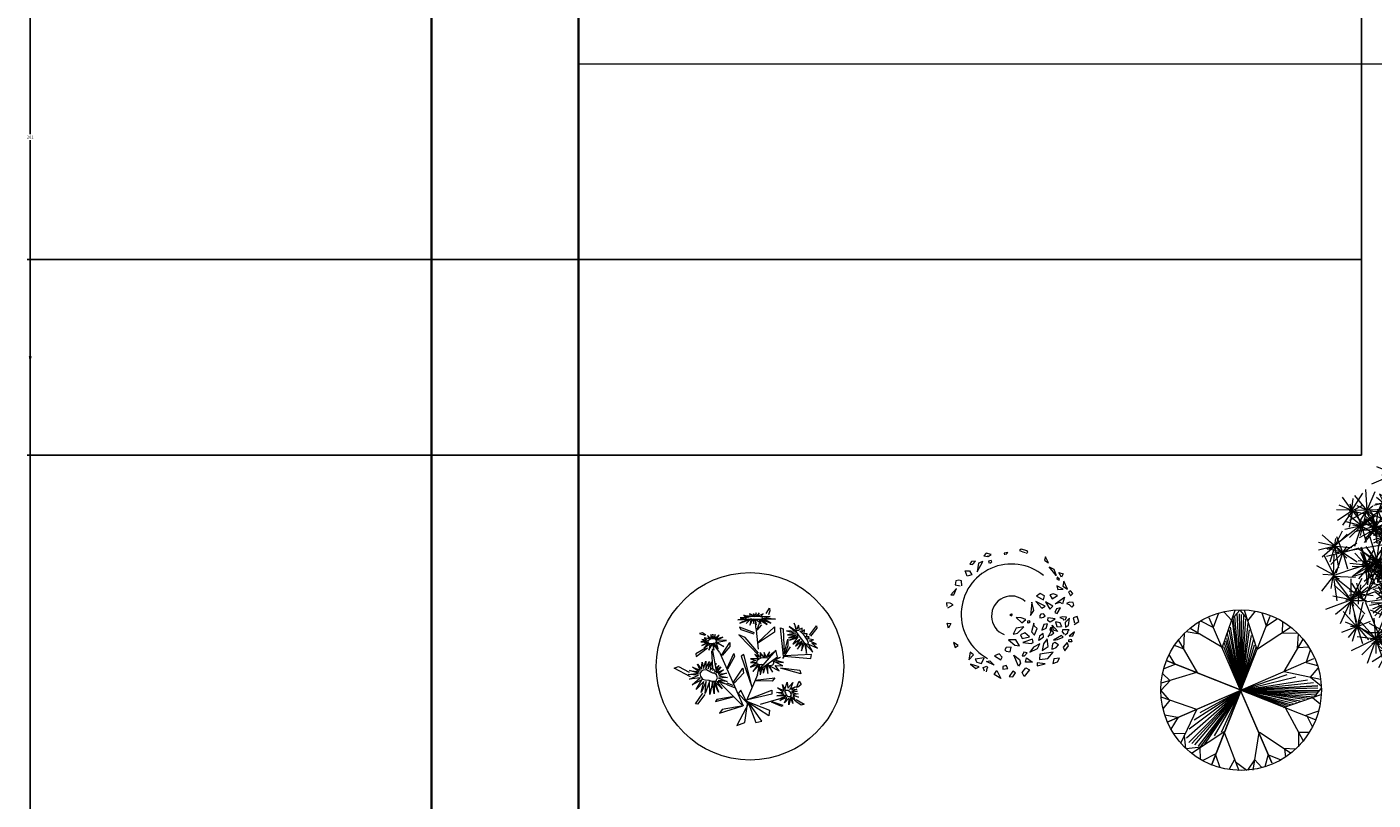
# Model space of a CAD drawing. Units: inches. Extents: x 8049 to 8459, y 820 to 1350.
# Tile 7 of 25: x 8050 to 8132, y 905 to 952. Entities that reach past the tile are written whole.
import ezdxf

# ---------------------------------------------------------------- set-up
doc = ezdxf.new("R2010")
doc.units = ezdxf.units.IN
doc.header["$MEASUREMENT"] = 0
for name, color, linetype, lineweight in [('A-ANNO-DIMS', 2, 'Continuous', 18), ('A-FLOR-STRS', 7, 'Continuous', 25), ('C-SITE-WALL', 7, 'Continuous', 35), ('L-PLNT-BEDS', 94, 'Continuous', 18), ('zelen', 69, 'Continuous', 13)]:
    doc.layers.add(name, color=color, linetype=linetype, lineweight=lineweight)
doc.styles.get("Standard").update_dxf_attribs({"font": 'arial.ttf'})
doc.dimstyles.get("Standard").update_dxf_attribs({"dimtxt": 0.18, "dimasz": 0.18, "dimexe": 0.18, "dimexo": 0.0625, "dimgap": 0.09, "dimtad": 0, "dimtih": 1, "dimtoh": 1, "dimdec": 4, "dimzin": 0, "dimdsep": 46, "dimtxsty": 'Standard', "dimcen": 0.09, "dimadec": 0, "dimazin": 0, "dimtfac": 1, "dimtdec": 4, "dimtofl": 0, "dimtmove": 0, "dimatfit": 3, "dimfxl": 1, "dimtolj": 1, "dimtzin": 0, "dimarcsym": 0})

# ---------------------------------------------------------------- blocks, each defined once
blk = doc.blocks.new('z_07')
for p, q in [((85.3, 280.8), (103, 308.6)), ((105.8, 294.2), (97.8, 273.4)), ((103, 308.6), (105.8, 294.2)), ((-21, 251.8), (-63.9, 246.3)), ((-63.9, 246.3), (-10.6, 249.9)), ((-10.6, 249.9), (-53.8, 228)), ((-53.8, 228), (-0.5, 249)), ((-17.8, 259.4), (-52, 257.4)), ((-52, 257.4), (-21, 251.8)), ((-33.4, 271.7), (-17.8, 259.4)), ((-5.4, 260.2), (-33.4, 271.7)), ((-20.7, 227.5), (5.4, 252.6)), ((-0.5, 249), (-20.7, 227.5)), ((-17.3, 268.5), (-5.4, 260.2)), ((0.4, 263.9), (-17.3, 268.5)), ((-2, 279), (0.4, 263.9)), ((16.1, 266.2), (-2, 279)), ((5.4, 252.6), (-0.2, 218.2)), ((-0.2, 218.2), (16.1, 251.8)), ((6.4, 274.5), (16.1, 266.2)), ((23.4, 266.3), (6.4, 274.5)), ((16.1, 251.8), (19.1, 227.4)), ((19, 279.6), (23.4, 266.3)), ((27.9, 266.9), (19, 279.6)), ((19.1, 227.4), (25, 251.4)), ((25, 251.4), (33.2, 219.8)), ((33.4, 283.2), (27.9, 266.9)), ((33.5, 194.3), (28.4, 231.3)), ((31.7, 250.6), (59.3, 226.6)), ((33.2, 219.8), (31.7, 250.6)), ((34.5, 265), (33.4, 283.2)), ((47.8, 284), (34.5, 265)), ((61.7, 219.6), (36.6, 191.4)), ((37.5, 194.8), (51.1, 228.1)), ((43.1, 265.9), (47.8, 284)), ((70.3, 277.4), (43.1, 265.9)), ((48.1, 248.2), (90.3, 221.2)), ((59.3, 226.6), (48.1, 248.2)), ((55.3, 262.3), (70.3, 277.4)), ((107.1, 264.9), (55.3, 262.3)), ((57.3, 249.7), (110, 229.2)), ((90.3, 221.2), (57.3, 249.7)), ((67.6, 251), (135.2, 249.3)), ((68.5, 256.1), (107.1, 264.9)), ((135.2, 249.3), (68.5, 256.1)), ((110, 229.2), (72.3, 251.5)), ((234, 228.4), (245.3, 186.3)), ((248.2, 196), (234, 228.4)), ((256.8, 219), (248.2, 196)), ((261.8, 195.5), (256.8, 219)), ((-251.2, 177.7), (-267.6, 173.3)), ((-267.6, 173.3), (-239.8, 164.3)), ((-233.4, 165.2), (-251.2, 177.7)), ((-243.6, 151.8), (-226, 137.3)), ((-216.2, 145.1), (-243.6, 151.8)), ((-225.7, 163.4), (-216.2, 145.1)), ((-208.5, 145.4), (-225.7, 163.4)), ((-208.7, 144.6), (-219.5, 136.6)), ((-198.7, 146.1), (-208.7, 144.6)), ((-207.9, 168.2), (-208.5, 145.4)), ((-197.8, 147.3), (-207.9, 168.2)), ((-188, 145.4), (-198.7, 146.1)), ((-196.5, 169.7), (-197.8, 147.3)), ((-192.3, 148.3), (-196.5, 169.7)), ((-185.4, 169.2), (-192.3, 148.3)), ((-185.1, 144.1), (-188, 145.4)), ((-184.1, 147.7), (-185.4, 169.2)), ((-179.1, 137.8), (-185.1, 144.1)), ((-164.3, 164.9), (-184.1, 147.7)), ((-179.3, 144.6), (-164.3, 164.9)), ((-144.4, 155), (-179.3, 144.6)), ((-177.3, 138.3), (-144.4, 155)), ((-58.7, 166.4), (50.5, 53.3)), ((-25.8, 153.4), (-58.7, 166.4)), ((-56, 207.7), (-48.9, 194.5)), ((23.9, 176.8), (-56, 207.7)), ((-48.9, 194.5), (20.9, 173)), ((44.9, 70.5), (-25.8, 153.4)), ((33.4, 191.9), (44, 90.1)), ((129.1, 181.5), (39.1, 121.3)), ((43.1, 127.7), (129.4, 208.7)), ((129.4, 208.7), (129.1, 181.5)), ((161.2, 204.4), (175.2, 197.9)), ((177.8, 54.5), (161.2, 204.4)), ((175.2, 197.9), (181.3, 66.4)), ((181.3, 66.4), (199.9, 143.5)), ((193.5, 188), (242.1, 176.2)), ((242, 184.3), (193.5, 188)), ((242.1, 176.2), (198.4, 166.1)), ((198.4, 166.1), (251.1, 167.3)), ((199.9, 143.5), (200.9, 108.9)), ((251.1, 167.3), (203.7, 151)), ((203.7, 151), (254, 160.4)), ((207.2, 210.7), (242, 184.3)), ((245.3, 186.3), (207.2, 210.7)), ((254, 160.4), (209.5, 138.3)), ((209.5, 138.3), (249.1, 150.4)), ((253.9, 156.5), (226.3, 116.7)), ((226.3, 116.7), (263.8, 143.7)), ((263.8, 143.7), (241.3, 106.4)), ((246.2, 187.2), (245.4, 181.5)), ((245.4, 181.5), (251.2, 171.8)), ((254.4, 190.4), (246.2, 187.2)), ((251.2, 171.8), (258.8, 160.8)), ((261.3, 189.2), (254.4, 190.4)), ((258.8, 160.8), (271.1, 146.1)), ((276.9, 201.7), (261.8, 195.5)), ((277.1, 175.7), (263.7, 186.3)), ((271.1, 146.1), (284.2, 130.2)), ((276.6, 182.8), (276.9, 201.7)), ((289.7, 193.6), (276.6, 182.8)), ((290.7, 160), (277.1, 175.7)), ((287, 171.3), (289.7, 193.6)), ((302.8, 171.8), (287, 171.3)), ((298.2, 149.9), (290.7, 160)), ((305.4, 138.6), (298.2, 149.9)), ((299, 156), (302.8, 171.8)), ((314, 156.8), (299, 156)), ((307.2, 145.4), (314, 156.8)), ((335.8, 139.8), (307.2, 145.4)), ((316.3, 165), (351.8, 213.8)), ((354.7, 202.6), (321.1, 159.3)), ((351.8, 213.8), (354.7, 202.6)), ((-235.3, 96.4), (-287.1, 65.9)), ((-285.8, 52.5), (-224.8, 98.6)), ((-260.9, 130.5), (-225.2, 126.2)), ((-228.7, 129.8), (-260.9, 130.5)), ((-255.4, 142.2), (-228.7, 129.8)), ((-226, 137.3), (-255.4, 142.2)), ((-254.6, 110.2), (-218.2, 126.3)), ((-225.2, 126.2), (-254.6, 110.2)), ((-218.2, 126.3), (-244.5, 95.4)), ((-244.5, 95.4), (-211, 120.2)), ((-219.5, 136.6), (-223.8, 129.5)), ((-223.8, 129.5), (-220.3, 123.5)), ((-220.3, 123.5), (-214.4, 120.6)), ((-211, 120.2), (-218.7, 86)), ((-218.7, 86), (-199, 119.8)), ((-214.4, 120.6), (-204.4, 121.7)), ((-204.6, 81.4), (-199.5, -9.8)), ((-204.4, 121.7), (-194.8, 122.3)), ((-199, 119.8), (-192.3, 84.8)), ((-175.3, -35.1), (-198.7, 92.4)), ((-194.8, 122.3), (-183.9, 124.5)), ((-192.3, 84.8), (-189.8, 119.4)), ((-189.8, 119.4), (-168.3, 91.9)), ((-161, 75.8), (-186.5, 108.1)), ((-183.9, 124.5), (-175.3, 127)), ((-179.8, 129.8), (-139.5, 105.2)), ((-168.3, 91.9), (-179.8, 129.8)), ((-177.1, 133.3), (-179.1, 137.8)), ((-177.5, 126.2), (-176.4, 128.6)), ((-139.5, 105.2), (-177.5, 124.5)), ((-124, 136.2), (-177.3, 138.3)), ((-176.4, 128.6), (-177.1, 133.3)), ((-173.3, 127.9), (-124, 136.2)), ((-161, 75.8), (-35.7, -210.4)), ((-153, 56.3), (-106.3, 126)), ((-106.9, 105.8), (-148.5, 57.6)), ((-106.3, 126), (-106.9, 105.8)), ((137.7, 84.7), (43.3, -23)), ((53.9, 72.9), (55.8, 46.8)), ((74.4, 46.6), (53.9, 72.9)), ((75.8, 72.7), (74.4, 46.6)), ((86.1, 47.7), (75.8, 72.7)), ((102.6, 76.8), (86.1, 47.7)), ((98.7, 50.4), (102.6, 76.8)), ((125.5, 74.7), (98.7, 50.4)), ((121.6, 66.3), (125.5, 74.7)), ((146.5, 51), (137.7, 84.7)), ((213, 103.6), (171.4, 40.8)), ((200.9, 108.9), (186.6, 68.8)), ((241.3, 106.4), (272.2, 133.8)), ((272.2, 133.8), (251.6, 91.4)), ((251.6, 91.4), (277.6, 125.4)), ((277.6, 125.4), (273.2, 82.7)), ((273.2, 82.7), (288.2, 124.6)), ((284.2, 130.2), (299.9, 116.2)), ((288.2, 124.6), (300.3, 67.6)), ((298.3, 113.8), (333.6, 74.1)), ((300.3, 67.6), (298.3, 113.8)), ((299.9, 116.2), (309.5, 123)), ((309.5, 123), (305.4, 138.6)), ((310, 116.8), (357.4, 96.4)), ((333.6, 74.1), (310, 116.8)), ((315.5, 135.5), (335.8, 139.8)), ((352.4, 118.2), (315.5, 135.5)), ((327.7, 122.6), (352.4, 118.2)), ((357.4, 96.4), (327.7, 122.6)), ((-287.1, 65.9), (-285.8, 52.5)), ((-278.8, 11), (-256.7, -14.8)), ((-264.2, -20.1), (-278.8, 11)), ((-256.7, -14.8), (-253.9, 22.7)), ((-253.9, 22.7), (-246.6, -11.2)), ((-246.6, -11.2), (-233.9, 26.9)), ((-233.9, 26.9), (-234.7, -14.3)), ((-234.7, -14.3), (-215.8, 24.7)), ((-215.8, 24.7), (-221.2, -12.7)), ((-221.2, -12.7), (-204.3, 24.2)), ((-204.3, 24.2), (-211.6, -17)), ((-183.3, 9.2), (-177.1, 15.7)), ((-182.9, 5.9), (-177.1, 15.7)), ((-179.2, -7.1), (-163.5, 4.7)), ((-177.8, -14.9), (-163.5, 4.7)), ((-121, -10), (-85.7, 67.7)), ((-81.5, 51.1), (-118.8, -15.9)), ((-85.7, 67.7), (-81.5, 51.1)), ((-32.2, 63.2), (-46.9, 53.3)), ((-46.9, 53.3), (9.1, -108.7)), ((7.2, -97), (-32.2, 63.2)), ((44.7, 39.2), (2.2, 38.8)), ((2.2, 38.8), (28.3, 31)), ((37.5, 20.3), (2.2, -5.3)), ((2.2, -5.3), (43.4, 11.4)), ((28.3, 31), (2.4, 19.3)), ((2.4, 19.3), (37.5, 20.3)), ((43.4, 11.4), (15.2, -28)), ((15.2, -28), (47.4, 4.5)), ((25.4, 62.8), (44.7, 39.2)), ((55.8, 46.8), (25.4, 62.8)), ((36.9, 28.9), (34.9, 20.5)), ((34.9, 20.5), (37.2, 13.9)), ((46.1, 37.3), (36.9, 28.9)), ((37.2, 13.9), (45.9, 11)), ((39.1, -45), (47.8, 1.4)), ((44.9, -22.6), (146.5, 51)), ((45.9, 11), (63.1, 9.1)), ((57.5, 43.2), (46.1, 37.3)), ((52.7, -13), (51.9, 8.7)), ((71.6, 45.6), (57.5, 43.2)), ((69.3, 8.1), (63.1, 9.1)), ((64.2, 2), (65.3, 8.2)), ((65.3, 8.2), (66.2, 4.8)), ((82.3, 4.4), (69.2, -36.7)), ((83, 45.7), (71.6, 45.6)), ((93.9, 43.8), (83, 45.7)), ((84.4, 6), (93.9, -38.4)), ((87.1, 6.1), (91, 5.8)), ((91, 5.8), (107, 4.7)), ((99.9, 41.6), (93.9, 43.8)), ((93.9, -38.4), (94.9, 9.1)), ((94.9, 9.1), (118.4, -31.9)), ((103.9, 1.8), (153.8, -23.7)), ((118.4, -31.9), (103.9, 1.8)), ((107, 4.7), (120.6, 8.6)), ((119.3, 31.3), (122.2, 29)), ((120.6, 8.6), (127.4, 21)), ((127.4, 21), (122.2, 29)), ((127.5, 26.1), (177.4, 19.7)), ((173.6, 2.2), (127.5, 26.1)), ((130.2, 33), (162.1, 48.8)), ((177.4, 19.7), (130.2, 33)), ((132.6, 41), (162.1, 48.8)), ((133.7, 4.9), (173.6, 2.2)), ((153.8, -23.7), (133.7, 4.9)), ((179.2, 54.2), (322.4, 41)), ((325.5, 62.5), (181.8, 56.3)), ((322.4, 41), (325.5, 62.5)), ((-401.9, -9.6), (-379.5, -0.2)), ((-316.3, -55.6), (-401.9, -9.6)), ((-379.5, -0.2), (-321.8, -31.6)), ((-327.2, -42.6), (-273.5, -37.2)), ((-273.3, -46.2), (-327.2, -42.6)), ((-321.4, -67.4), (-273.3, -46.2)), ((-264.4, -61.8), (-321.4, -67.4)), ((-320.8, -21.7), (-269.2, -29.5)), ((-273.5, -37.2), (-320.8, -21.7)), ((-306.3, -97.5), (-264.4, -61.8)), ((-304.1, -4.5), (-264.2, -20.1)), ((-269.2, -29.5), (-304.1, -4.5)), ((-199.2, -7.5), (-212.9, -21.9)), ((-195.5, -15.5), (-199.7, -22.6)), ((-194, -18.3), (-199.7, -22.6)), ((-199.5, -9.8), (-175.3, -35.1)), ((-185.4, -25.3), (-188.2, -29.1)), ((-185.3, -26.8), (-188.2, -29.1)), ((-177.3, -20.7), (-154.6, -3.3)), ((-154.6, -3.3), (-177, -34.7)), ((-177, -34.7), (-141.4, -17.9)), ((-141.4, -17.9), (-169.7, -41.4)), ((-169.7, -41.4), (-123.8, -36.5)), ((-119, -59.3), (-167.6, -62.1)), ((-167.6, -62.1), (-120.9, -80.4)), ((-123.8, -36.5), (-165.8, -50.2)), ((-165.8, -50.2), (-119, -59.3)), ((-87.9, -84.4), (-38.6, -9.6)), ((-35.2, -35.6), (-84.2, -89.8)), ((-38.6, -9.6), (-35.2, -35.6)), ((39.1, -45), (-19, -181)), ((27.1, -73.7), (132.1, -61.1)), ((52.9, -17.7), (53.9, -45.1)), ((62.8, -9.7), (53.9, -45.1)), ((67.9, -6), (69.2, -36.7)), ((132.1, -61.1), (117.7, -79.1)), ((269.4, -39.7), (161.2, -10.1)), ((162.5, -8), (265, -20.8)), ((265, -20.8), (269.4, -39.7)), ((-254.9, -71.5), (-306.3, -97.5)), ((-289.3, -199.2), (-249.4, -141.8)), ((-286.2, -122.5), (-254.9, -71.5)), ((-244.5, -81.1), (-286.2, -122.5)), ((-232, -80.6), (-259.7, -139.6)), ((-259.7, -139.6), (-244.5, -81.1)), ((-214.2, -80.4), (-237.3, -144.1)), ((-237.3, -144.1), (-232, -80.6)), ((-212.8, -150.3), (-214.2, -80.4)), ((-198.5, -83.3), (-212.8, -150.3)), ((-190.2, -145.4), (-198.5, -83.3)), ((-189.5, -85.3), (-190.2, -145.4)), ((-167.7, -136.5), (-189.5, -85.3)), ((-186.3, -82.5), (-167.7, -136.5)), ((-147.8, -118.8), (-186.3, -82.5)), ((-175.8, -80), (-147.8, -118.8)), ((-121.6, -96.5), (-175.8, -80)), ((-168, -75), (-121.6, -96.5)), ((-120.9, -80.4), (-168, -75)), ((-157.2, -91.9), (-44.1, -203.7)), ((-90.2, -102.6), (-121.5, -89.6)), ((-80.5, -114), (-118, -100.6)), ((-49.1, -127), (-62.3, -145)), ((-12.6, -198.5), (-49.1, -127)), ((-17.1, -177), (116.1, -126.4)), ((117.7, -79.1), (28.4, -76.2)), ((116.1, -126.4), (115.5, -148.1)), ((140.7, -138.3), (175.2, -136.5)), ((180.5, -147.4), (140.7, -138.3)), ((145.9, -113.6), (179.1, -127.9)), ((175.2, -136.5), (145.9, -113.6)), ((171.4, -95.7), (184.9, -122.5)), ((179.1, -127.9), (171.4, -95.7)), ((184.9, -122.5), (196.7, -84.2)), ((196.7, -84.2), (200.9, -115.8)), ((200.9, -115.8), (227.1, -86.7)), ((208.5, -121.7), (241.2, -108.7)), ((227.1, -86.7), (212.5, -123.9)), ((241.2, -108.7), (219.9, -125.3)), ((219.9, -125.3), (247.4, -121.9)), ((247.4, -121.9), (220.2, -134.6)), ((220.2, -134.6), (249.2, -132)), ((249.2, -132), (220.8, -140.2)), ((220.8, -140.2), (255.6, -145.2)), ((247, -112.9), (259.8, -79.1)), ((270.8, -96.5), (251.1, -111.6)), ((259.8, -79.1), (270.8, -96.5)), ((-278.3, -200.8), (-289.3, -199.2)), ((-239.8, -150.1), (-278.3, -200.8)), ((-183.8, -187.5), (-90.1, -161.1)), ((-176, -176.8), (-183.8, -187.5)), ((-94.3, -161.3), (-176, -176.8)), ((-161, -249.4), (-37.6, -210)), ((-36.1, -210), (-148.2, -228.8)), ((-6.3, -194.1), (-70.4, -313.3)), ((-62.3, -145), (-16, -191.1)), ((-28, -297.6), (-12.6, -198.5)), ((-19.5, -184.8), (103, -231.9)), ((115.5, -148.1), (-12.7, -177.2)), ((-10.4, -192.3), (30.8, -297.4)), ((99.4, -263.3), (-10.4, -192.3)), ((62.9, -291.3), (-6.3, -194.1)), ((151.6, -173.6), (53.5, -202.8)), ((112.5, -188.5), (167, -212.2)), ((176.5, -207.3), (117.7, -188.9)), ((142.6, -156), (180.5, -147.4)), ((189.3, -156.2), (142.6, -156)), ((151.6, -173.6), (179.7, -161.5)), ((158.9, -181.7), (189.3, -156.2)), ((194.8, -166.3), (158.9, -181.7)), ((167, -212.2), (176.5, -207.3)), ((183.3, -192.9), (194.8, -166.3)), ((207.6, -167.1), (183.3, -192.9)), ((215.9, -165.8), (205.3, -205.2)), ((205.3, -205.2), (207.6, -167.1)), ((227.9, -197.8), (215.9, -165.8)), ((219.6, -162.5), (227.9, -197.8)), ((240.6, -184.8), (219.6, -162.5)), ((255.6, -145.2), (226.2, -150.6)), ((226.2, -150.6), (256.4, -164)), ((228.7, -155.9), (240.6, -184.8)), ((256.4, -164), (228.7, -155.9)), ((271.8, -206.6), (243.8, -186.4)), ((245.2, -175.7), (287.5, -200.6)), ((287.5, -200.6), (271.8, -206.6)), ((-148.2, -228.8), (-161, -249.4)), ((103, -231.9), (99.4, -263.3)), ((-70.4, -313.3), (-28, -297.6)), ((30.8, -297.4), (62.9, -291.3))]:
    blk.add_line(p, q)
for points in [[(26.3, 263.3), (22.9, 264.5), (12.8, 264.3), (2.9, 262.7), (-9.7, 260.6), (-20.2, 257.5), (-25.1, 254.7), (-20.2, 251.3), (-1.3, 250.6), (16.7, 251.1), (38.2, 250.3), (52.3, 250.3), (67.9, 252.7), (64.7, 261.3), (50.6, 264.3), (36.5, 264.6), (22.8, 262.9)], [(-211.4, -28.6), (-222.1, -23.5), (-231.1, -19.5), (-248.3, -20.6), (-259.5, -28.3), (-265.7, -37.4), (-262.3, -51.8), (-252.4, -67.8), (-238.9, -71.3), (-218.5, -74.3), (-202.3, -78), (-182.1, -79.6), (-172.2, -60.6), (-177.8, -44.4), (-191.8, -35.5)], [(-211.4, -28.6), (-208.4, -29.2), (-206.4, -30.7), (-204.3, -31.6), (-202.2, -33.1), (-199.4, -34.2), (-195.7, -35.1), (-191.8, -35.8), (-191.8, -35.5)], [(214.6, -141.2), (213.8, -137.6), (210, -133.3), (202.5, -128.4), (190.3, -129), (183.7, -134.2), (187.4, -141.4), (190.6, -149.7), (197.3, -159.1), (207.6, -160.4), (215.4, -159.3), (220.7, -151.3), (216.9, -142.9), (213.1, -138.2)]]:
    blk.add_lwpolyline(points)
blk.add_circle((0, 0), 496.9)
blk = doc.blocks.new('T40C')
for p, q in [((-0.1219, 0.4263), (-0.1133, 0.5002)), ((-0.0016, 0.4444), (-0.055, 0.5069)), ((-0.0016, 0.0138), (-0.0016, 0.5115)), ((-0.0016, 0.5115), (-0.0016, -0.4769)), ((-0.0016, 0.4364), (0.0585, 0.5048)), ((0.1041, 0.4402), (0.0754, 0.5038)), ((-0.2, 0.2178), (-0.2513, 0.4459)), ((-0.2374, 0.3843), (-0.221, 0.4586)), ((-0.1327, 0.438), (-0.2166, 0.4607)), ((-0.0047, 0.2984), (-0.1711, 0.4799)), ((-0.0016, 0.2889), (0.1386, 0.4896)), ((-0.0016, 0.0138), (0.1054, 0.4378)), ((-0.0016, 0.0138), (0.1166, 0.4328)), ((0.0011, 0.0164), (0.1417, 0.4349)), ((0.0011, 0.0164), (0.1801, 0.4343)), ((0.0011, 0.0164), (0.161, 0.432)), ((0.0979, 0.4313), (0.1806, 0.4751)), ((0.2217, 0.4068), (0.1848, 0.4759)), ((0.2091, 0.2244), (0.2252, 0.4573)), ((0.2208, 0.3933), (0.2879, 0.4166)), ((0.3508, 0.3661), (-0.3487, -0.3333)), ((0.0011, 0.0164), (-0.3443, 0.3618)), ((-0.3443, 0.3618), (0.3464, -0.329)), ((-0.3045, 0.3219), (-0.313, 0.3998)), ((-0.2369, 0.3817), (-0.2976, 0.4118)), ((-0.0016, 0.0138), (0.2033, 0.4135)), ((-0.0016, 0.0138), (0.0852, 0.4075)), ((-0.0016, 0.0138), (0.2072, 0.3567)), ((0.0011, 0.0164), (0.3508, 0.3661)), ((0.0011, 0.0164), (0.0491, 0.3369)), ((0.2979, 0.3132), (0.3134, 0.399)), ((-0.377, 0.2509), (-0.4492, 0.2275)), ((-0.2034, 0.2144), (-0.4335, 0.2627)), ((-0.3838, 0.2523), (-0.4084, 0.2975)), ((-0.3055, 0.3229), (-0.3893, 0.3231)), ((-0.0016, 0.0138), (0.1989, 0.2926)), ((0.0011, 0.0164), (0.0175, 0.3021)), ((0.3008, 0.3162), (0.3801, 0.3306)), ((0.3847, 0.2335), (0.4047, 0.2984)), ((-0.4278, 0.1246), (-0.4601, 0.209)), ((-0.0016, 0.0138), (0.1836, 0.2378)), ((0.2092, 0.2254), (0.4418, 0.2362)), ((0.3861, 0.2336), (0.4597, 0.1963)), ((0.3915, 0.2339), (0.3982, 0.2342)), ((0.4263, 0.1181), (0.4586, 0.1989)), ((-0.4281, 0.1249), (-0.4899, 0.1006)), ((-0.2946, 0.0138), (-0.4744, 0.1635)), ((0.2937, 0.0138), (0.4738, 0.1555)), ((0.4291, 0.1204), (0.4873, 0.0978)), ((-0.4418, 0.0138), (-0.4967, 0.0634)), ((-0.4277, 0.0138), (-0.4952, -0.0443)), ((0.4953, 0.0138), (-0.4939, 0.0138)), ((-0.2846, 0.0167), (-0.4721, -0.1432)), ((-0.0016, 0.0138), (-0.4477, -0.1559)), ((-0.0016, 0.0138), (-0.4464, -0.1312)), ((-0.0016, 0.0138), (-0.4422, -0.1429)), ((-0.0016, 0.0138), (-0.4379, -0.1735)), ((-0.0016, 0.0138), (-0.4328, -0.1117)), ((-0.0016, 0.0138), (-0.4324, -0.1862)), ((-0.4324, -0.1862), (-0.0016, 0.0138)), ((-0.0016, 0.0138), (-0.4146, -0.0968)), ((-0.0016, 0.0138), (-0.4013, -0.1946)), ((-0.0016, 0.0138), (-0.3864, -0.0775)), ((-0.0016, 0.0138), (-0.3647, -0.0593)), ((-0.0016, 0.0138), (-0.3588, -0.1967)), ((-0.0016, 0.0138), (-0.3309, -0.0302)), ((-0.0016, 0.0138), (-0.3156, -0.0151)), ((-0.0016, 0.0138), (-0.3007, -0.0042)), ((-0.0016, 0.0138), (-0.2917, 0.0059)), ((-0.0016, 0.0138), (-0.2861, -0.1863)), ((-0.0016, 0.0138), (-0.2311, -0.181)), ((-0.0016, 0.0138), (-0.0528, -0.0021)), ((-0.0016, 0.0138), (-0.0528, -0.0021)), ((-0.0016, 0.0138), (0.0011, 0.0164)), ((-0.0016, 0.0138), (0.4953, 0.0138)), ((-0.0016, 0.0138), (0.0088, -0.2669)), ((-0.0016, 0.0138), (0.0243, -0.2768)), ((-0.0016, 0.0138), (0.0408, -0.3033)), ((-0.0016, 0.0138), (0.0625, -0.3241)), ((-0.0016, 0.0138), (0.0872, -0.3518)), ((-0.0016, 0.0138), (0.1104, -0.3878)), ((-0.0016, 0.0138), (0.1339, -0.4064)), ((-0.0016, 0.0138), (0.1521, -0.4202)), ((-0.0016, 0.0138), (0.1669, -0.4211)), ((-0.0016, 0.0138), (0.1801, -0.4202)), ((-0.0016, 0.0138), (0.1959, -0.4202)), ((-0.0016, 0.0138), (0.2013, -0.3955)), ((-0.0016, 0.0138), (0.2072, -0.3832)), ((-0.0016, 0.0138), (0.2062, -0.3647)), ((-0.0016, 0.0138), (0.2018, -0.3233)), ((-0.0016, 0.0138), (0.2038, -0.3052)), ((-0.0016, 0.0138), (0.2044, -0.2809)), ((-0.0016, 0.0138), (0.1983, -0.2504)), ((-0.0016, 0.0138), (0.197, -0.2334)), ((-0.0016, 0.0138), (0.2007, -0.2173)), ((-0.0016, 0.0138), (0.1959, -0.1959)), ((0.285, 0.0138), (0.4722, -0.133)), ((0.2917, 0.0138), (0.3747, 0.0138)), ((0.4315, 0.0138), (0.491, 0.0679)), ((0.4349, 0.0169), (0.4927, -0.0276)), ((-0.0528, -0.0021), (-0.4551, -0.1664)), ((-0.0528, -0.0021), (-0.3463, -0.045)), ((-0.4294, -0.1068), (-0.4874, -0.0863)), ((-0.4387, -0.1147), (-0.459, -0.1779)), ((0.4191, -0.0914), (0.4833, -0.0909)), ((0.4217, -0.0934), (0.4533, -0.184)), ((-0.3712, -0.2192), (-0.4529, -0.1923)), ((-0.2066, -0.1906), (-0.4335, -0.23)), ((-0.3712, -0.2192), (-0.3953, -0.2872)), ((-0.2067, -0.1914), (-0.2414, -0.4204)), ((0.2042, -0.1867), (0.2149, -0.4325)), ((0.2071, -0.1897), (0.4318, -0.2236)), ((0.3628, -0.2132), (0.4476, -0.1967)), ((0.3755, -0.2151), (0.3928, -0.2871)), ((-0.3126, -0.2938), (-0.3837, -0.3016)), ((-0.3124, -0.2971), (-0.3082, -0.3761)), ((-0.0016, -0.2596), (-0.1424, -0.4599)), ((-0.0016, -0.2565), (0.16, -0.4525)), ((0.3007, -0.2833), (0.3874, -0.2905)), ((0.3008, -0.2851), (0.3017, -0.3787)), ((-0.2322, -0.3601), (-0.2902, -0.3882)), ((-0.2315, -0.3548), (-0.2033, -0.4394)), ((-0.1046, -0.4061), (-0.1917, -0.4425)), ((-0.1086, -0.4118), (-0.0869, -0.4727)), ((-0.0016, -0.4144), (-0.047, -0.4779)), ((-0.0016, -0.4109), (0.0515, -0.477)), ((0.1172, -0.4006), (0.0947, -0.4728)), ((0.1259, -0.4112), (0.1857, -0.4428)), ((0.2123, -0.3741), (0.1875, -0.442)), ((0.212, -0.3667), (0.2724, -0.3967))]:
    blk.add_line(p, q)
blk.add_circle((-0.0016, 0.0138), 0.496)
blk = doc.blocks.new('z_66')
for p, q in [((-254, 399.9), (-283.6, 397.7)), ((-272.8, 380.7), (-254, 399.9)), ((-176.4, 458.5), (-191.7, 438.6)), ((-191.7, 438.6), (-165.6, 433.5)), ((-139.2, 449.4), (-176.4, 458.5)), ((-165.6, 433.5), (-163.6, 441.1)), ((-165.6, 433.5), (-165.6, 433.5)), ((-161.1, 434.6), (-139.2, 449.4)), ((-138.9, 404.9), (-156.9, 400.2)), ((-156.9, 400.2), (-153.8, 385.4)), ((-133.3, 394.8), (-138.9, 404.9)), ((-13.6, 463.6), (-42.5, 459.2)), ((-42.5, 459.2), (-39.3, 446.9)), ((-30.3, 449.4), (-13.6, 463.6)), ((83.2, 488.9), (72.7, 477.7)), ((72.7, 477.7), (96.4, 469.7)), ((129.8, 476.2), (83.2, 488.9)), ((96.4, 469.7), (114.5, 463.9)), ((114.5, 463.9), (114.5, 463.9)), ((120.4, 457.8), (134, 464.6)), ((134, 464.6), (129.8, 476.2)), ((265.2, 432.1), (258.2, 407.5)), ((258.2, 407.5), (287.4, 387.2)), ((258.2, 407.5), (281.9, 388.6)), ((287.4, 387.2), (265.2, 432.1)), ((-330.3, 328.9), (-298.6, 327.1)), ((-316, 288.8), (-330.3, 328.9)), ((-298.6, 327.1), (-280.8, 297.1)), ((-283.6, 397.7), (-297.2, 378.2)), ((-297.2, 378.2), (-277.7, 376)), ((-277.7, 376), (-272.8, 380.7)), ((-241.9, 321.7), (-199.1, 397.3)), ((-231.4, 383.6), (-241.9, 321.7)), ((-199.1, 397.3), (-231.4, 383.6)), ((-148.6, 384.7), (-133.3, 394.8)), ((281.9, 388.6), (281.9, 388.6)), ((344.2, 293.1), (292, 357.2)), ((292, 357.2), (326.8, 341.2)), ((326.8, 341.2), (344.2, 293.1)), ((383.1, 281.9), (364.4, 316.3)), ((364.4, 316.3), (394.6, 305.1)), ((394.6, 305.1), (383.1, 281.9)), ((-399.2, 252.6), (-405.8, 224)), ((-405.8, 224), (-368.2, 216.4)), ((-377.9, 259.1), (-399.2, 252.6)), ((-358.4, 254), (-377.9, 259.1)), ((-368.2, 216.4), (-368.2, 216.4)), ((-356, 217.5), (-358.4, 254)), ((-280.8, 297.1), (-316, 288.8)), ((348, 215.7), (356, 188.9)), ((395.3, 193.2), (348, 215.7)), ((350.8, 280.8), (348.7, 270.3)), ((348.7, 270.3), (358.8, 264.5)), ((369.2, 266.7), (350.8, 280.8)), ((358.8, 264.5), (358.8, 264.5)), ((363.3, 256.6), (369.2, 266.7)), ((400.9, 251.9), (393.9, 214.6)), ((393.9, 214.6), (426.6, 192.2)), ((426.6, 192.2), (400.9, 251.9)), ((-396.4, 196.1), (-438.1, 150.2)), ((-438.1, 150.2), (-414.8, 150.9)), ((-414.8, 150.9), (-396.4, 196.1)), ((193.1, 101.3), (238, 52.1)), ((261.7, 66.6), (193.1, 101.3)), ((225.2, 159.9), (197, 140.8)), ((197, 140.8), (249.5, 113.6)), ((256.8, 142.6), (225.2, 159.9)), ((249.5, 113.6), (256.8, 142.6)), ((323.6, 157.8), (297.5, 149.8)), ((297.5, 149.8), (314.6, 119.4)), ((314.6, 119.4), (352.9, 145.5)), ((352.9, 145.5), (323.6, 157.8)), ((336.9, 84.3), (405.8, 131.7)), ((356, 188.9), (395.3, 193.2)), ((405.8, 131.7), (389.8, 82.1)), ((450, 180.6), (434.3, 171.2)), ((434.3, 171.2), (449.6, 142.6)), ((449.6, 142.6), (467.7, 160.3)), ((467.7, 160.3), (450, 180.6)), ((-468.4, 91.6), (-466.3, 62.6)), ((-441.6, 89), (-468.4, 91.6)), ((-466.3, 62.6), (-466.3, 62.6)), ((-458.3, 53.9), (-421.1, 76)), ((-421.1, 76), (-441.6, 89)), ((11.8, 6.2), (0, 0)), ((0, 0), (12.2, -6.9)), ((12.2, -6.9), (19.1, 2.9)), ((19.1, 2.9), (15.7, 5.8)), ((164.3, 94.8), (154.2, -2.2)), ((154.2, -2.2), (178.9, 33.3)), ((178.9, 33.3), (164.3, 94.8)), ((229, 7.2), (223.1, -2.5)), ((250.6, 9.8), (229, 7.2)), ((238, 52.1), (261.7, 66.6)), ((263.4, -5.4), (250.6, 9.8)), ((265.2, 98.8), (297.2, 42.7)), ((318.8, 66.2), (265.2, 98.8)), ((297.2, 42.7), (294.1, 53.6)), ((297.2, 42.7), (318.8, 66.2)), ((347.3, 45.2), (332.7, 18.1)), ((332.7, 18.1), (350.8, 10.9)), ((372.7, 93), (336.9, 84.3)), ((376.9, 52.5), (347.3, 45.2)), ((350.8, 10.9), (376.9, 52.5)), ((389.8, 82.1), (372.7, 93)), ((441.6, 95.9), (420.7, 86.5)), ((420.7, 86.5), (440.2, 78.5)), ((440.2, 78.5), (459.7, 59.7)), ((470.5, 93.7), (441.6, 95.9)), ((459.7, 59.7), (459.7, 59.7)), ((463.2, 57.9), (474, 73.5)), ((474, 73.5), (470.5, 93.7)), ((-464.2, -59.3), (-436.4, -62.6)), ((-454.5, -96.3), (-464.2, -59.3)), ((-436.4, -62.6), (-454.5, -96.3)), ((47.7, -96.6), (24, -141.9)), ((104.1, -87.9), (47.7, -96.6)), ((84.6, -21.7), (48, -17)), ((48, -17), (90.1, -58.3)), ((56, -133.9), (104.1, -87.9)), ((119.4, -32.9), (84.6, -21.7)), ((90.1, -58.3), (119.4, -32.9)), ((131.9, -44.9), (130.2, -52.5)), ((130.2, -52.5), (132.9, -59.3)), ((146.5, -42.3), (131.9, -44.9)), ((138.2, -56.8), (151, -51)), ((151, -51), (146.5, -42.3)), ((177.8, -59), (160.1, -123.8)), ((181, -80.3), (177.8, -59)), ((202.2, -100.6), (181, -80.3)), ((223.1, -2.5), (222.7, -20.6)), ((222.7, -20.6), (234.2, -18.1)), ((233.2, -19.9), (249.9, -15.9)), ((234.2, -18.1), (234.2, -18.1)), ((252.6, -70.9), (237.7, -112.9)), ((237.7, -112.9), (269.7, -98.4)), ((249.9, -15.9), (263.4, -5.4)), ((278.4, -64), (252.6, -70.9)), ((269.7, -98.4), (278.4, -64)), ((282.9, -21.3), (279.1, -39.1)), ((279.1, -39.1), (298.6, -50.3)), ((302.1, -22.8), (282.9, -21.3)), ((301.7, -95.5), (297.9, -112.2)), ((298.6, -50.3), (335.8, -28.6)), ((310.8, -91.9), (301.7, -95.5)), ((335.8, -28.6), (302.1, -22.8)), ((307.6, -106), (310.8, -91.9)), ((314.2, -74.2), (356.7, -123)), ((323.3, -111.1), (314.2, -74.2)), ((339, -51), (347.7, -84.3)), ((374.1, -56.8), (339, -51)), ((347.7, -84.3), (379.7, -88.3)), ((393.6, -13), (371, -17)), ((371, -17), (383.5, -23.5)), ((386.3, -87.9), (374.1, -56.8)), ((379.7, -88.3), (379.7, -88.3)), ((383.5, -23.5), (396.7, -28.9)), ((420, -15.9), (393.6, -13)), ((396.7, -28.9), (398.5, -35.5)), ((398.5, -35.5), (399.5, -35.8)), ((410.3, -38), (420, -15.9)), ((442, -22.4), (411.3, -55.4)), ((411.3, -55.4), (412.7, -90.8)), ((412.7, -90.8), (436, -77.1)), ((436, -77.1), (442, -22.4)), ((499.7, -10.9), (468.8, -19.9)), ((468.8, -19.9), (478.8, -58.6)), ((477.5, -70.2), (510.9, -47)), ((478.8, -58.6), (478.8, -58.6)), ((510.9, -47), (499.7, -10.9)), ((44.5, -184.2), (-10.8, -184.9)), ((-10.8, -184.9), (36.9, -222.2)), ((24, -141.9), (56, -133.9)), ((71, -229.1), (44.5, -184.2)), ((111.4, -132.8), (78.3, -146.2)), ((78.3, -146.2), (92.2, -174.1)), ((92.2, -174.1), (145.1, -162.1)), ((168.1, -178.4), (96.7, -202.6)), ((145.1, -162.1), (111.4, -132.8)), ((160.1, -123.8), (179.6, -146.6)), ((173, -203.4), (168.1, -178.4)), ((179.6, -146.6), (183.7, -145.5)), ((183.7, -145.5), (202.2, -100.6)), ((220.6, -157), (212.6, -186)), ((212.6, -186), (219.2, -183.5)), ((219.2, -183.5), (249.2, -162.1)), ((247.1, -135.7), (220.6, -157)), ((249.2, -162.1), (247.1, -135.7)), ((277.4, -176.2), (250.2, -212.4)), ((283.3, -233.8), (277.4, -176.2)), ((291.6, -145.8), (281.2, -161.8)), ((281.2, -161.8), (293, -152.7)), ((304.5, -123), (291.6, -145.8)), ((293, -152.7), (308.3, -145.8)), ((297.9, -112.2), (304.5, -123)), ((325.4, -132.4), (307.6, -106)), ((308.3, -145.8), (325.4, -132.4)), ((356.7, -123), (323.3, -111.1)), ((382.5, -152.7), (323.3, -187.4)), ((323.3, -187.4), (353.9, -182)), ((353.9, -182), (396.7, -164.3)), ((356.7, -123), (356.7, -123)), ((356.7, -123), (356.7, -123)), ((396.7, -164.3), (382.5, -152.7)), ((391.2, -110), (388.4, -125.6)), ((388.4, -125.6), (402.3, -140.8)), ((391.2, -110), (393.2, -108.6)), ((441.3, -110), (391.2, -110)), ((402.3, -140.8), (402.3, -140.8)), ((407.9, -145.5), (427, -133.5)), ((427, -133.5), (432.9, -115.8)), ((432.9, -115.8), (441.3, -110)), ((438.5, -183.8), (456.2, -179.1)), ((438.5, -197.6), (438.5, -183.8)), ((458.7, -199), (438.5, -197.6)), ((480.9, -124.5), (439.2, -156)), ((439.2, -156), (467.7, -153.4)), ((456.2, -179.1), (458.7, -199)), ((467.7, -153.4), (480.9, -124.5)), ((-417.9, -204.1), (-405.1, -239.6)), ((-382.8, -226.5), (-417.9, -204.1)), ((-405.1, -239.6), (-382.8, -226.5)), ((-295.1, -275), (-304.2, -331.5)), ((-304.2, -331.5), (-269, -296)), ((-269, -296), (-295.1, -275)), ((-80, -288), (-112.4, -302.5)), ((-56.7, -311.6), (-80, -288)), ((-26.4, -240.3), (-37.6, -258.4)), ((-37.6, -258.4), (-25.8, -268.5)), ((10.1, -237.7), (-26.4, -240.3)), ((-25.8, -268.5), (2.4, -273.2)), ((-25.8, -268.5), (-25.8, -268.5)), ((-25.8, -268.5), (-25.8, -268.5)), ((2.4, -273.2), (10.1, -237.7)), ((30.6, -297.1), (72.7, -329.3)), ((64, -379.6), (30.6, -297.1)), ((36.9, -222.2), (71, -229.1)), ((105.1, -276.1), (91.9, -303.6)), ((96.7, -202.6), (157.6, -211.3)), ((128.8, -280.4), (105.1, -276.1)), ((108.6, -301.4), (128.8, -280.4)), ((175.4, -237.7), (149.6, -276.1)), ((149.6, -276.1), (204.3, -246.8)), ((157.6, -211.3), (173, -203.4)), ((223.8, -212.4), (175.4, -237.7)), ((204.3, -246.8), (223.8, -212.4)), ((223.8, -290.2), (221.3, -330)), ((322.2, -275), (223.8, -290.2)), ((250.2, -212.4), (240.1, -262.4)), ((240.1, -262.4), (283.3, -233.8)), ((282.2, -321.7), (322.2, -275)), ((314.6, -228.7), (311.8, -252.6)), ((311.8, -252.6), (320.5, -249.3)), ((318.4, -212.1), (314.6, -228.7)), ((334.1, -203.7), (318.4, -212.1)), ((320.5, -249.3), (342.8, -241.4)), ((360.2, -221.1), (334.1, -203.7)), ((342.8, -241.4), (360.2, -221.1)), ((425.3, -204.5), (396.7, -238.5)), ((396.7, -238.5), (409.2, -264.2)), ((409.2, -264.2), (434.3, -228)), ((434.3, -228), (425.3, -204.5)), ((-292, -364.4), (-252, -395.5)), ((-228.3, -383.9), (-292, -364.4)), ((-191.1, -317.4), (-256.8, -326.4)), ((-256.8, -326.4), (-245.7, -350.3)), ((-252, -395.5), (-228.3, -383.9)), ((-245.7, -350.3), (-209.8, -360.4)), ((-209.8, -360.4), (-191.1, -317.4)), ((-197.3, -388.3), (-171.2, -377.8)), ((-188.3, -416.9), (-197.3, -388.3)), ((-169.5, -396.6), (-174.7, -420.5)), ((-172.6, -344.9), (-146.9, -338.7)), ((-114.8, -372.7), (-172.6, -344.9)), ((-171.2, -377.8), (-166, -391.5)), ((-166, -391.5), (-169.5, -396.6)), ((-146.9, -338.7), (-114.8, -372.7)), ((-112.4, -302.5), (-67.5, -331.8)), ((-67.5, -331.8), (-56.7, -311.6)), ((-27.8, -374.5), (-52.9, -381.8)), ((-52.9, -381.8), (-50.8, -402)), ((-50.8, -402), (-15.3, -396.2)), ((-15.3, -396.2), (-27.8, -374.5)), ((79.3, -357.9), (64, -379.6)), ((72.7, -329.3), (79.3, -357.9)), ((91.9, -303.6), (108.6, -301.4)), ((91.9, -424.8), (119, -391.5)), ((117.3, -348.8), (124.2, -317.7)), ((168.8, -349.9), (117.3, -348.8)), ((119, -391.5), (146.9, -406.4)), ((124.2, -317.7), (168.8, -349.9)), ((201.8, -355), (202.2, -376.3)), ((261, -362.2), (201.8, -355)), ((202.2, -376.3), (261, -362.2)), ((221.3, -330), (282.2, -321.7)), ((325.7, -323.9), (318.4, -360.1)), ((318.4, -360.1), (354.3, -346.3)), ((368.9, -319.2), (325.7, -323.9)), ((354.3, -346.3), (368.9, -319.2)), ((-174.7, -420.5), (-174.7, -420.5)), ((-116.2, -441.1), (-96.4, -411.8)), ((-65.8, -470.8), (-116.2, -441.1)), ((-96.4, -411.8), (-65.8, -470.8)), ((21.6, -417.2), (-4.5, -455.6)), ((-4.5, -455.6), (21.6, -458.1)), ((42.1, -428.8), (21.6, -417.2)), ((21.6, -458.1), (42.1, -428.8)), ((106.8, -455.6), (91.9, -424.8)), ((146.9, -406.4), (106.8, -455.6))]:
    blk.add_line(p, q)
for centre, radius, start, end in [((11.8, 6.2), 372.3, 50.21175, 241.51848), ((12.2, -6.9), 147.8, 46.76113, 248.90672)]:
    blk.add_arc(centre, radius, start, end)
blk = doc.blocks.new('z_96')
for p, q in [((-279.8, 149.9), (-254.2, 304.5)), ((-277.5, 143.8), (-209, 319.2)), ((0.6, 181.7), (29.5, 299.6)), ((-282.5, 143.4), (-440.4, 263.7)), ((-279.3, 139.9), (-326.8, 270.9)), ((-276.5, 141.1), (-146.8, 221.3)), ((-9.6, 182.8), (-129.6, 222.9)), ((1.7, 182.4), (-92.5, 262.1)), ((-2.3, 183.5), (-55.4, 292.1)), ((3.6, 188.7), (58.7, 265.3)), ((5.7, 184.9), (91.8, 284.8)), ((393.4, 89.6), (354, 209.2)), ((395.6, 94.6), (438.6, 246.5)), ((-283.2, 138.5), (-471.2, 114.9)), ((-292.1, 134.2), (-430.8, 180.4)), ((-279.1, 142.3), (-397.9, 16.9)), ((-285.6, 136.6), (-375, 92.2)), ((-277.6, 139.7), (-313.4, -1.1)), ((-279.1, 135.4), (-307.4, 99.5)), ((-280.1, 150.3), (-304, 174)), ((-278.4, 130.6), (-221.9, 40)), ((-277.5, 137.2), (-129.1, 19.3)), ((-17.8, -5.6), (-274.7, 141.8)), ((-263.2, 140.3), (-131, 113.5)), ((-260.4, 142.3), (-97.9, 156.1)), ((-5.7, 186.4), (-99.8, 114.3)), ((-4.6, 181.6), (-86.6, 72.3)), ((-4.6, -3.2), (0.8, 176.4)), ((-0.6, 184.6), (125.7, 194.4)), ((1.5, 182.8), (69.9, 77.5)), ((9.8, 182.3), (88, 114.6)), ((393.4, 89.6), (284.7, 153.1)), ((393.4, 89.6), (479.1, 181.8)), ((393.4, 89.6), (514.5, 123.6)), ((-74.7, -24.6), (-111.9, 37.5)), ((-71.7, -35.5), (-42.1, 65.4)), ((0, 0), (389.1, 84.4)), ((164.1, -89.9), (142.7, 11.7)), ((163.4, -89), (238.9, 7.6)), ((393.4, 89.6), (273.9, 50.1)), ((393.4, 89.6), (293.9, 12.5)), ((391.3, 83.5), (363.2, 41.9)), ((393.4, 89.6), (493.5, 13.4)), ((393.4, 89.6), (516.7, 64.5)), ((393.4, 89.6), (442.6, -26.2)), ((409.2, 93.4), (456.4, 89)), ((-237.5, -199.4), (-267, -22)), ((-10.4, -6), (-235.7, -205.3)), ((-234, -202.3), (-196.3, -40.6)), ((-75, -39.2), (-157.1, -75.4)), ((-74, -33), (-152.4, -40.5)), ((-65.2, -32.9), (-135.5, -11.4)), ((-76.2, -35.8), (-103.5, -105.8)), ((-80, -28.7), (-89.9, -20)), ((-16, -6.1), (-74.7, -37.4)), ((-72.5, -35.1), (-71.9, -112)), ((-70.4, -41.1), (3.7, -57.1)), ((-69.9, -39.6), (-38.4, -102.6)), ((-68.1, -28.4), (-55.8, -19.3)), ((-5, -18.9), (163.8, -91.6)), ((167.1, -94.6), (37.3, -175)), ((161.1, -92.4), (74, -95.2)), ((159.3, -86.3), (85.5, -28.7)), ((163.4, -86.5), (137.7, -55.7)), ((164.5, -93.4), (157.3, -141.4)), ((160.4, -93), (267.6, -148.2)), ((164.2, -92.2), (234.3, -170.2)), ((165.3, -92), (295.7, -74)), ((166.9, -90.5), (187.1, -100.1)), ((167, -88.4), (276, -24.7)), ((168.3, -88.4), (194, -71.5)), ((-237.4, -199.3), (-392.1, -169)), ((-242.3, -196.3), (-391.5, -241.3)), ((-242.2, -199.4), (-329.5, -310.3)), ((-246.4, -194), (-283.1, -163.8)), ((-231, -196), (-205.2, -161.9)), ((163.6, -101.8), (119, -170.9)), ((167, -104.1), (188, -212.9)), ((-241, -201.7), (-259.1, -277.3)), ((-242.2, -201.7), (-47.9, -207.3)), ((-236.2, -200.9), (-139.2, -306.8)), ((-230.8, -205.8), (-146.5, -236))]:
    blk.add_line(p, q)
blk = doc.blocks.new('сосна 1')
for p, rotation in [((317.7, 388.3), 121.1570021628385), ((-412.6, 386.5), 205.4822314301707), ((-117.1, 122.3), 55.05972244949475), ((-351.5, 121.7), 257.3134436407499), ((-136.5, 361.1), 177.7388340989747), ((285.8, 9.1), 60.73020616460848), ((-343.1, -101.5), 57.88453704712605), ((-143.1, -5.5), 121.1570021628385), ((234.4, -65.1), 73.8676290404427), ((-274, 161.3), 177.7388340989747), ((173.8, 17), 349.7944254651076), ((98.1, -4.6), 177.7388340989747), ((326.9, 45.9), 177.7388340989747), ((-502.4, -282.3), 279.7984529833926), ((-175.3, -367), 63.19571700542104), ((-48.9, -393.6), 342.5348703671633), ((260.9, -458.6), 13.72293452966709)]:
    blk.add_blockref('z_96', p, dxfattribs=dict(rotation=rotation))
blk = doc.blocks.new('*D50')
at = {"layer": 'A-ANNO-DIMS', "color": 0, "lineweight": -2, "transparency": 16777216}
for p, q in [((8083.335, 1045.871), (8049.617, 1045.871)), ((8049.797, 1045.691), (8049.797, 945.553)), ((8049.797, 845.051), (8049.797, 945.189)), ((8074.335, 844.871), (8049.617, 844.871))]:
    blk.add_line(p, q, dxfattribs=at)
at = {"layer": 'A-ANNO-DIMS', "color": 0, "transparency": 16777216}
for points in [[(8049.767, 1045.691), (8049.827, 1045.691), (8049.797, 1045.871)], [(8049.767, 845.051), (8049.827, 845.051), (8049.797, 844.871)]]:
    blk.add_solid(points, dxfattribs=at)
at = {"layer": 'Defpoints', "color": 0, "transparency": 16777216}
for p in [(8049.797, 1045.871), (8083.397, 1045.871), (8074.397, 844.871)]:
    blk.add_point(p, dxfattribs=at)
at = {"layer": 'A-ANNO-DIMS', "color": 0, "transparency": 16777216, "insert": (8049.797, 945.371), "char_height": 0.18, "attachment_point": 5}
blk.add_mtext('\\A1;201', dxfattribs=at)
blk = doc.blocks.new('*D59')
at = {"layer": 'A-ANNO-DIMS', "color": 0, "lineweight": -2, "transparency": 16777216}
for p, q in [((8083.397, 925.933), (8083.397, 1349.651)), ((8083.577, 1349.471), (8107.175, 1349.471)), ((8131.217, 1349.471), (8107.62, 1349.471)), ((8131.397, 925.933), (8131.397, 1349.651))]:
    blk.add_line(p, q, dxfattribs=at)
at = {"layer": 'A-ANNO-DIMS', "color": 0, "transparency": 16777216}
for points in [[(8083.577, 1349.501), (8083.577, 1349.441), (8083.397, 1349.471)], [(8131.217, 1349.501), (8131.217, 1349.441), (8131.397, 1349.471)]]:
    blk.add_solid(points, dxfattribs=at)
at = {"layer": 'Defpoints', "color": 0, "transparency": 16777216}
for p in [(8131.397, 1349.471), (8083.397, 925.871), (8131.397, 925.871)]:
    blk.add_point(p, dxfattribs=at)
at = {"layer": 'A-ANNO-DIMS', "color": 0, "transparency": 16777216, "insert": (8107.397, 1349.471), "char_height": 0.18, "attachment_point": 5}
blk.add_mtext('\\A1;48', dxfattribs=at)
blk = doc.blocks.new('*D60')
at = {"layer": 'A-ANNO-DIMS', "color": 0, "lineweight": -2, "transparency": 16777216}
for p, q in [((8083.335, 937.871), (8049.617, 937.871)), ((8049.797, 937.691), (8049.797, 932.051)), ((8049.797, 926.051), (8049.797, 931.69)), ((8083.335, 925.871), (8049.617, 925.871))]:
    blk.add_line(p, q, dxfattribs=at)
at = {"layer": 'A-ANNO-DIMS', "color": 0, "transparency": 16777216}
for points in [[(8049.767, 937.691), (8049.827, 937.691), (8049.797, 937.871)], [(8049.767, 926.051), (8049.827, 926.051), (8049.797, 925.871)]]:
    blk.add_solid(points, dxfattribs=at)
at = {"layer": 'Defpoints', "color": 0, "transparency": 16777216}
for p in [(8049.797, 937.871), (8083.397, 937.871), (8083.397, 925.871)]:
    blk.add_point(p, dxfattribs=at)
at = {"layer": 'A-ANNO-DIMS', "color": 0, "transparency": 16777216, "insert": (8049.797, 931.871), "char_height": 0.18, "attachment_point": 5}
blk.add_mtext('\\A1;12', dxfattribs=at)
blk = doc.blocks.new('*D70')
at = {"layer": 'A-ANNO-DIMS', "color": 0, "lineweight": -2, "transparency": 16777216}
for p, q in [((8083.397, 1045.808), (8083.397, 820.091)), ((8137.397, 1045.808), (8137.397, 820.091)), ((8083.577, 820.271), (8110.179, 820.271)), ((8137.217, 820.271), (8110.616, 820.271))]:
    blk.add_line(p, q, dxfattribs=at)
at = {"layer": 'A-ANNO-DIMS', "color": 0, "transparency": 16777216}
for points in [[(8083.577, 820.301), (8083.577, 820.241), (8083.397, 820.271)], [(8137.217, 820.301), (8137.217, 820.241), (8137.397, 820.271)]]:
    blk.add_solid(points, dxfattribs=at)
at = {"layer": 'Defpoints', "color": 0, "transparency": 16777216}
for p in [(8083.397, 1045.871), (8137.397, 1045.871), (8083.397, 820.271)]:
    blk.add_point(p, dxfattribs=at)
at = {"layer": 'A-ANNO-DIMS', "color": 0, "transparency": 16777216, "insert": (8110.397, 820.271), "char_height": 0.18, "attachment_point": 5}
blk.add_mtext('\\A1;54', dxfattribs=at)
blk = doc.blocks.new('*D76')
at = {"layer": 'A-ANNO-DIMS', "color": 0, "lineweight": -2, "transparency": 16777216}
for p, q in [((8083.397, 1054.808), (8083.397, 820.091)), ((8299.397, 1054.808), (8299.397, 820.091)), ((8083.577, 820.271), (8191.107, 820.271)), ((8299.217, 820.271), (8191.688, 820.271))]:
    blk.add_line(p, q, dxfattribs=at)
at = {"layer": 'A-ANNO-DIMS', "color": 0, "transparency": 16777216}
for points in [[(8083.577, 820.301), (8083.577, 820.241), (8083.397, 820.271)], [(8299.217, 820.301), (8299.217, 820.241), (8299.397, 820.271)]]:
    blk.add_solid(points, dxfattribs=at)
at = {"layer": 'Defpoints', "color": 0, "transparency": 16777216}
for p in [(8083.397, 1054.871), (8299.397, 1054.871), (8299.397, 820.271)]:
    blk.add_point(p, dxfattribs=at)
at = {"layer": 'A-ANNO-DIMS', "color": 0, "transparency": 16777216, "insert": (8191.397, 820.271), "char_height": 0.18, "attachment_point": 5}
blk.add_mtext('\\A1;216', dxfattribs=at)
blk = doc.blocks.new('*D88')
at = {"layer": 'A-ANNO-DIMS', "color": 0, "lineweight": -2, "transparency": 16777216}
for p, q in [((8083.397, 1162.808), (8083.397, 820.091)), ((8139.397, 1162.808), (8139.397, 820.091)), ((8083.577, 820.271), (8111.179, 820.271)), ((8139.217, 820.271), (8111.616, 820.271))]:
    blk.add_line(p, q, dxfattribs=at)
at = {"layer": 'A-ANNO-DIMS', "color": 0, "transparency": 16777216}
for points in [[(8083.577, 820.301), (8083.577, 820.241), (8083.397, 820.271)], [(8139.217, 820.301), (8139.217, 820.241), (8139.397, 820.271)]]:
    blk.add_solid(points, dxfattribs=at)
at = {"layer": 'Defpoints', "color": 0, "transparency": 16777216}
for p in [(8083.397, 1162.871), (8139.397, 1162.871), (8139.397, 820.271)]:
    blk.add_point(p, dxfattribs=at)
at = {"layer": 'A-ANNO-DIMS', "color": 0, "transparency": 16777216, "insert": (8111.397, 820.271), "char_height": 0.18, "attachment_point": 5}
blk.add_mtext('\\A1;56', dxfattribs=at)

msp = doc.modelspace()

# ---------------------------------------------------------------- linework, layer by layer
at = {"layer": 'A-FLOR-STRS'}
for p, q in [((8131.3974, 1045.8706), (8131.3974, 925.8706)), ((8083.3974, 937.8706), (8131.3974, 937.8706)), ((8083.3974, 925.8706), (8131.3974, 925.8706))]:
    msp.add_line(p, q, dxfattribs=at)
at = {"layer": 'C-SITE-WALL'}
for p, q in [((8074.3974, 1324.8706), (8074.3974, 844.8706)), ((8083.3974, 1315.8706), (8083.3974, 853.8706))]:
    msp.add_line(p, q, dxfattribs=at)
at = {"layer": 'L-PLNT-BEDS'}
msp.add_line((8083.3974, 949.8706), (8197.3974, 949.8706), dxfattribs=at)

# ---------------------------------------------------------------- block references
at = {"layer": 'zelen'}
for name, p, xscale, yscale, zscale in [('сосна 1', (8135.8007, 919.1777), 0.0082668533249786, 0.0082668533249786, 0.0082668533249786), ('z_66', (8109.8408, 916.073), 0.0082668533249786, 0.0082668533249786, 0.0082668533249786), ('z_07', (8093.9162, 912.9314), 0.0115605630918543, 0.0115605630918543, 0.0115605630918543)]:
    msp.add_blockref(name, p, dxfattribs=dict(at, xscale=xscale, yscale=yscale, zscale=zscale))
at = {"layer": 'zelen', "xscale": 9.920223989974332, "yscale": 9.920223989974332, "zscale": 9.920223989974332, "rotation": 158.4000000000004}
msp.add_blockref('T40C', (8124.0525, 911.6043), dxfattribs=at)

# ---------------------------------------------------------------- dimensions: what is measured, and where the dimension line sits
at = {"layer": 'A-ANNO-DIMS'}
for base, p1, p2, picture, middle in [((8131.3974, 1349.4706), (8083.3974, 925.8706), (8131.3974, 925.8706), '*D59', (8107.3974, 1349.4706)), ((8139.3974, 820.2706), (8083.3974, 1162.8706), (8139.3974, 1162.8706), '*D88', (8111.3974, 820.2706)), ((8299.3974, 820.2706), (8083.3974, 1054.8706), (8299.3974, 1054.8706), '*D76', (8191.3974, 820.2706)), ((8083.3974, 820.2706), (8137.3974, 1045.8706), (8083.3974, 1045.8706), '*D70', (8110.3974, 820.2706))]:
    dim = msp.add_linear_dim(base=base, p1=p1, p2=p2, dimstyle='Standard', override={"dimdec": 0, "dimlfac": 1, "dimrnd": 0, "dimzin": 0, "dimdsep": 46, "dimlunit": 2}, dxfattribs=at)
    dim.commit()
    dim.dimension.update_dxf_attribs({"geometry": picture, "text_midpoint": middle})
for base, p1, p2, picture, middle in [((8049.7974, 1045.8706), (8074.3974, 844.8706), (8083.3974, 1045.8706), '*D50', (8049.7974, 945.3706)), ((8049.7974, 937.8706), (8083.3974, 925.8706), (8083.3974, 937.8706), '*D60', (8049.7974, 931.8706))]:
    dim = msp.add_linear_dim(base=base, p1=p1, p2=p2, angle=90, dimstyle='Standard', override={"dimdec": 0, "dimlfac": 1, "dimrnd": 0, "dimzin": 0, "dimdsep": 46, "dimlunit": 2}, dxfattribs=at)
    dim.commit()
    dim.dimension.update_dxf_attribs({"geometry": picture, "text_midpoint": middle})

doc.saveas('drawing.dxf')
